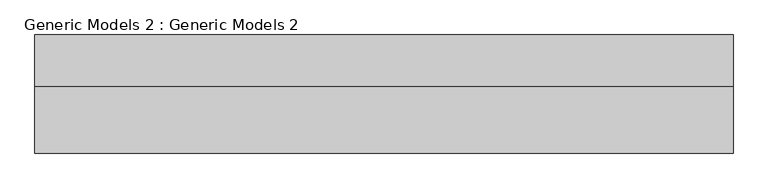
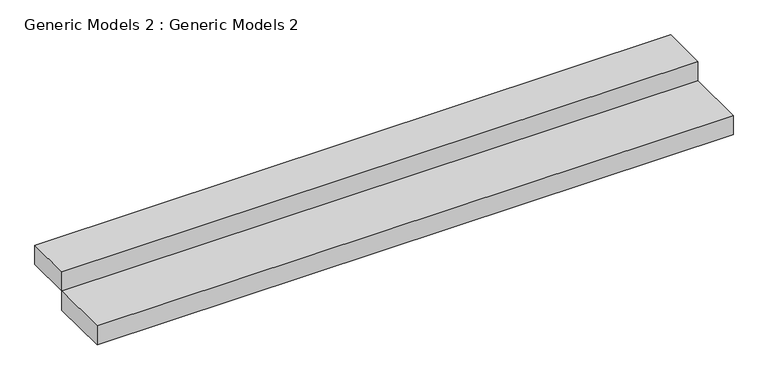
"""IFC4 building model written with IfcOpenShell, lengths in millimetres: proxy geometry, Generic Models 2 : Generic Models 2."""

from ifc_helpers import new_model, si_unit, frame, origin, origin_with_axes, place, context, project, spatial, polyline, outline, extrude, source, transform, mapped, element, save


def generic_models_2_generic_models_2_230f2d88(model_context):
    return source(origin(), model_context, "Body", "SweptSolid", [
        extrude(outline(polyline([(-15214.3530968, -17083.0021511), (-15214.3530968, -16164.71773), (-5613.1530968, -16164.71773), (-5613.1530968, -17083.0021511), (-15214.3530968, -17083.0021511)])), frame((0.0, 0.0, -304.8), z_axis=(0.0, 0.0, 1.0), x_axis=(1.0, 0.0, 0.0)), (0.0, 0.0, 1.0), 304.8),
        extrude(outline(polyline([(-5613.1530968, -15458.6370893), (-5613.1530968, -16164.71773), (-15214.3530968, -16164.71773), (-15214.3530968, -15458.6370893), (-5613.1530968, -15458.6370893)])), origin_with_axes(), (0.0, 0.0, 1.0), 304.8),
    ])


if __name__ == "__main__":
    model = new_model("IFC4")
    model_context = context("Model", 3, world=origin())
    ifc_project = project(units=[si_unit("LENGTHUNIT", "METRE", prefix="MILLI")], contexts=[model_context])
    site = spatial("IfcSite", under=ifc_project)
    building = spatial("IfcBuilding", under=site)
    placement = place(None, origin())
    generic_models_2_generic_models_2_shape = generic_models_2_generic_models_2_230f2d88(model_context)
    element("IfcBuildingElementProxy", 1, Name="Generic Models 2 : Generic Models 2", ObjectType="Generic Models 2 : Generic Models 2", at=placement, inside=building, context=model_context, shape_type="MappedRepresentation", body=[
        mapped(generic_models_2_generic_models_2_shape, transform((0.0, 0.0, 0.0), x_axis=(1.0, 0.0, 0.0), y_axis=(0.0, 1.0, 0.0), z_axis=(0.0, 0.0, 1.0))),
    ])
    save(model, "model.ifc")
